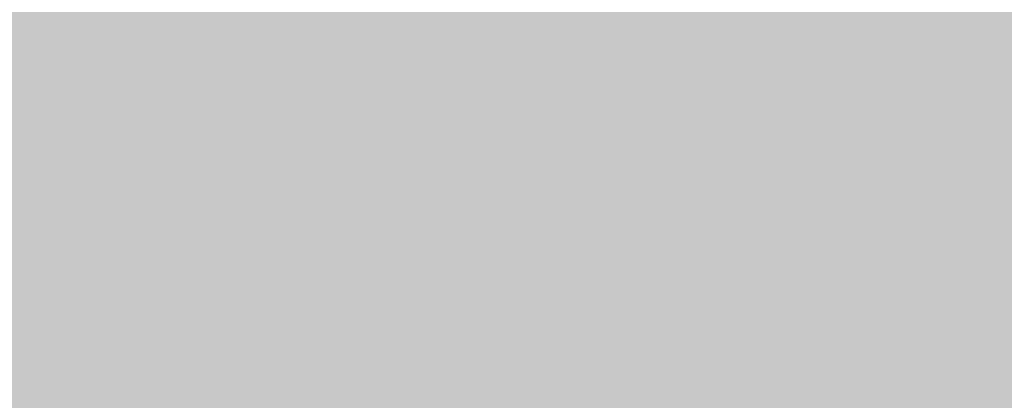
# Model space of a CAD drawing. Units: feet. Extents: x 3168 to 4724, y 827 to 1477.
# Tile 56 of 256: x 3273.139442 to 3273.143144, y 1099.01485 to 1099.016281. Entities that reach past the tile are written whole.
import ezdxf

# ---------------------------------------------------------------- set-up
doc = ezdxf.new("R2010")
doc.units = ezdxf.units.FT
doc.layers.add('A-ELEV', color=7, linetype='Continuous', lineweight=35)
doc.layers.add('A-ELEV-PATT', color=8, linetype='Continuous', lineweight=13)

msp = doc.modelspace()

# ---------------------------------------------------------------- hatches: boundary and pattern name
at = {"layer": 'A-ELEV-PATT'}
h = msp.add_hatch(color=256, dxfattribs=at)
h.dxf.hatch_style = 1
edge = h.paths.add_edge_path()
edge.add_ellipse((3552.9057615, 979.2201412), major_axis=(36.7449243, 0), ratio=0.4848484848, start_angle=0, end_angle=360)
edge = h.paths.add_edge_path()
edge.add_ellipse((3559.8916366, 929.2522824), major_axis=(36.7449243, 0), ratio=0.4848484848, start_angle=0, end_angle=360)
edge = h.paths.add_edge_path()
edge.add_line((3299.3168105, 1198.606081), (3479.9167135, 1198.606081))
edge.add_line((3479.9167135, 1198.606081), (3479.9167135, 1209.8685704))
edge.add_spline(control_points=[(3479.9167135, 1209.8685704), (3464.3011571, 1209.8685704), (3448.6856007, 1209.8685704), (3410.949139, 1209.8685704), (3388.8282339, 1209.8685704), (3355.6468761, 1209.8685704), (3344.5864235, 1209.8685704), (3327.9957446, 1209.8685704), (3322.4655183, 1209.8685704), (3314.1701788, 1209.8685704), (3311.4050657, 1209.8685704), (3307.257396, 1209.8685704), (3305.8748394, 1209.8685704), (3303.8010045, 1209.8685704), (3303.1097262, 1209.8685704), (3302.0728088, 1209.8685704), (3301.7271697, 1209.8685704), (3301.2087109, 1209.8685704), (3301.0358914, 1209.8685704), (3300.776662, 1209.8685704), (3300.6902522, 1209.8685704), (3300.5606376, 1209.8685704), (3300.5174327, 1209.8685704), (3300.4526253, 1209.8685704), (3300.4310229, 1209.8685704), (3300.3986192, 1209.8685704), (3300.387818, 1209.8685704), (3300.3662155, 1209.8685704), (3300.3456757, 1209.8685704), (3300.3455476, 1209.8685704), (3300.345505, 1209.8685704), (3300.3433041, 1209.8685704), (3300.341146, 1209.8685707), (3300.337909, 1209.8685714), (3300.33683, 1209.8685718), (3300.3339422, 1209.8685728), (3300.3321334, 1209.8685736), (3300.3255154, 1209.8685773), (3300.3207065, 1209.8685812), (3300.3109248, 1209.8685917), (3300.305952, 1209.8685984), (3300.2905113, 1209.8686233), (3300.2800452, 1209.8686461), (3300.2324255, 1209.868777), (3300.1952979, 1209.868954), (3299.9510684, 1209.8706077), (3299.7448244, 1209.8743259), (3299.4368271, 1209.8832566), (3299.3343894, 1209.8867924), (3299.181079, 1209.8929197), (3299.1300333, 1209.8950994), (3298.6522171, 1209.9168011), (3298.2294605, 1209.9457176), (3297.6016312, 1210.0023671), (3297.3934043, 1210.0234637), (3297.082652, 1210.058309), (3296.9793324, 1210.0704575), (3296.2929541, 1210.1548606), (3295.7181475, 1210.2433556), (3294.8687167, 1210.3988504), (3294.5876997, 1210.4544779), (3294.1693407, 1210.5433488), (3294.0304153, 1210.5738777), (3291.7071487, 1211.1012), (3289.6535901, 1211.8134353), (3285.7762586, 1213.5639876), (3283.9514101, 1214.6034778), (3280.512159, 1216.9800798), (3278.8972407, 1218.3175918), (3276.3799143, 1220.829489), (3275.4160415, 1221.9177379), (3274.0393421, 1223.7076996), (3273.5810428, 1224.3495346), (3273.1432283, 1225.0163162)], knot_values=[39.119033, 39.119033, 39.119033, 39.119033, 39.286353, 39.286353, 39.523379, 39.523379, 39.641892, 39.641892, 39.701148, 39.701148, 39.730777, 39.730777, 39.745591, 39.745591, 39.752998, 39.752998, 39.756701, 39.756701, 39.758553, 39.758553, 39.759479, 39.759479, 39.759942, 39.759942, 39.760173, 39.760173, 39.760289, 39.760289, 39.760405, 39.760405, 39.760463, 39.760463, 39.763389, 39.763389, 39.764851, 39.764851, 39.767304, 39.767304, 39.773825, 39.773825, 39.78057, 39.78057, 39.79477, 39.79477, 39.845194, 39.845194, 40.126715, 40.126715, 40.267476, 40.267476, 40.337856, 40.337856, 40.927023, 40.927023, 41.221606, 41.221606, 41.368898, 41.368898, 42.202622, 42.202622, 42.619485, 42.619485, 42.827916, 42.827916, 46.118323, 46.118323, 49.408731, 49.408731, 52.699139, 52.699139, 54.927489, 54.927489, 56.104228, 56.104228, 56.104228, 56.104228], weights=[1, 1, 1, 1, 1, 1, 1, 1, 1, 1, 1, 1, 1, 1, 1, 1, 1, 1, 1, 1, 1, 1, 1, 1, 1, 1, 1, 1, 1, 1, 1, 1, 1, 1, 1, 1, 1, 1, 1, 1, 1, 1, 1, 1, 1, 1, 1, 1, 1, 1, 1, 1, 1, 1, 1, 1, 1, 1, 1, 1, 1, 1, 1, 1, 1, 1, 1, 1, 1, 1, 1, 1, 1, 1], degree=3, periodic=0)
edge.add_line((3273.1432283, 1225.0163162), (3273.1432283, 1099.0163162))
edge.add_line((3273.1432283, 1099.0163162), (3299.3168105, 1099.0163162))
edge.add_line((3299.3168105, 1099.0163162), (3299.3168105, 1198.606081))
edge = h.paths.add_edge_path()
edge.add_line((3304.7584434, 1324.15806), (3479.9167135, 1324.15806))
edge.add_line((3479.9167135, 1324.15806), (3479.9167135, 1335.7146184))
edge.add_line((3479.9167135, 1335.7146184), (3269.1616284, 1335.7146184))
edge.add_spline(control_points=[(3269.1616284, 1335.7146184), (3264.0242315, 1335.7146184), (3258.364118, 1328.9581888), (3259.2643109, 1323.9002743)], knot_values=[0, 0, 0, 0, 15.412191, 15.412191, 15.412191, 15.412191], degree=3, periodic=0)
edge.add_line((3259.2643109, 1323.9002743), (3265.5168487, 1288.7691348))
edge.add_line((3265.5168487, 1288.7691348), (3275.2651026, 1261.5456259))
edge.add_line((3275.2651026, 1261.5456259), (3304.7584434, 1261.5456259))
edge.add_line((3304.7584434, 1261.5456259), (3304.7584434, 1324.15806))
h = msp.add_hatch(color=256, dxfattribs=at)
h.dxf.hatch_style = 1
h.paths.add_polyline_path([(3384.5252473, 1099.0163162), (3335.0291678, 1099.0163162), (3299.3168105, 1099.0163162), (3273.1432283, 1099.0163162), (3217.5653642, 1099.0163162), (3168.0692847, 827.1162598), (3335.0291678, 827.1162598)])

# ---------------------------------------------------------------- linework, layer by layer
at = {"layer": 'A-ELEV'}
msp.add_open_spline([(3808.5202001, 1099.0163162), (3808.5202001, 1141.413235), (3808.5202001, 1183.8101539), (3808.5202001, 1226.6353244), (3808.5202001, 1227.0635761), (3808.5202001, 1227.4918279), (3811.491871, 1248.9946729), (3814.463542, 1270.497518), (3817.4652299, 1292.2175635), (3817.4952467, 1292.434764), (3817.5252636, 1292.6519644), (3817.5728014, 1310.1067483), (3817.6203393, 1327.5615322), (3817.6678771, 1345.0163162), (3817.6678771, 1345.4579619), (3817.6678771, 1345.8996077), (3817.6678771, 1346.4560466), (3817.6678771, 1346.5708398), (3817.6678771, 1346.7528874), (3817.6678771, 1346.8201418), (3817.6678771, 1346.9348705), (3817.6678771, 1346.9823447), (3817.6678771, 1347.0385872), (3817.6678771, 1347.0473556), (3817.6678771, 1347.0736607), (3817.667877, 1347.0593025), (3817.6678766, 1347.0615455), (3817.6678764, 1347.0626669), (3817.6678754, 1347.0660311), (3817.6678743, 1347.0682738), (3817.6678701, 1347.0750012), (3817.667866, 1347.0794856), (3817.6678493, 1347.0929368), (3817.6678325, 1347.1019019), (3817.6677657, 1347.1287896), (3817.6676988, 1347.1467049), (3817.6674317, 1347.2004211), (3817.6671649, 1347.2361922), (3817.6661003, 1347.3433849), (3817.6650383, 1347.4146859), (3817.6608124, 1347.6280949), (3817.6566084, 1347.7697085), (3817.6399698, 1348.1924868), (3817.6235091, 1348.4715855), (3817.5590944, 1349.3000666), (3817.4961208, 1349.8405878), (3817.2554319, 1351.4241561), (3817.0263177, 1352.4287852), (3816.3068713, 1354.8889138), (3815.7437452, 1356.2687272), (3814.4639586, 1358.8192105), (3813.7464132, 1359.9909676), (3812.1958378, 1362.1723433), (3811.3622453, 1363.1821237), (3809.5888357, 1365.0690087), (3808.6488164, 1365.9461052), (3806.6542623, 1367.5796162), (3805.5997024, 1368.336154), (3803.3528906, 1369.7223272), (3802.1605354, 1370.352386), (3799.6008131, 1371.4535864), (3798.2326878, 1371.9254812), (3795.2800838, 1372.6346239), (3793.6931479, 1372.8720685), (3791.8694413, 1372.9264797), (3791.7408615, 1372.9292203), (3791.3533713, 1372.9341014), (3791.0927074, 1372.9329013), (3790.3041163, 1372.9150676), (3789.7695426, 1372.8841946), (3789.20919, 1372.8302363), (3789.1906217, 1372.8284241), (3789.1348916, 1372.8229123), (3789.097705, 1372.8191375), (3789.0484446, 1372.8140077), (3789.0364001, 1372.8127432), (3789.0002562, 1372.808918), (3788.9761468, 1372.8063255), (3788.9494049, 1372.8034042), (3788.9467858, 1372.8031177), (3788.9425667, 1372.8026552), (3788.9409669, 1372.8024797), (3788.9385718, 1372.8022166), (3788.9377765, 1372.8021292), (3788.9353908, 1372.8018669), (3788.8675349, 1372.7944024), (3788.7568665, 1372.7822285), (3788.7015323, 1372.7761415), (3788.5355297, 1372.7578805), (3788.4248612, 1372.7457065), (3788.092856, 1372.7091846), (3787.8715192, 1372.6848366), (3787.2075086, 1372.6117927), (3786.764835, 1372.5630968), (3785.436814, 1372.417009), (3784.5514666, 1372.3196171), (3781.8954246, 1372.0274416), (3780.1247299, 1371.8326579), (3774.8126458, 1371.2483067), (3771.2712564, 1370.8587393), (3760.6470883, 1369.6900371), (3753.5643095, 1368.9109022), (3732.3159732, 1366.5734977), (3718.1504157, 1365.015228), (3694.0067577, 1362.3593262), (3684.0286573, 1361.2616941), (3674.0505568, 1360.1640619), (3664.6006617, 1360.1640619), (3655.1507666, 1360.1640619), (3626.8010812, 1360.1640619), (3607.9012909, 1360.1640619), (3551.2019201, 1360.1640619), (3513.4023395, 1360.1640619), (3467.7251817, 1360.1640619), (3459.8476045, 1360.1640619), (3436.2148727, 1360.1640619), (3420.4597182, 1360.1640619), (3373.1942547, 1360.1640619), (3341.6839457, 1360.1640619), (3302.8481616, 1360.1640619), (3295.5226865, 1360.1640619), (3286.0382916, 1360.1640619), (3283.8793719, 1360.1640619), (3277.4026128, 1360.1640619), (3273.0847733, 1360.1640619), (3267.7328511, 1360.1640619), (3266.6987684, 1360.1640619), (3263.5965201, 1360.1640619), (3261.5283546, 1360.1640619), (3259.2369429, 1360.1640619), (3259.0136967, 1360.1640619), (3258.3439582, 1360.1640619), (3257.8974658, 1360.1640619), (3257.4309979, 1360.1640619), (3257.4110224, 1360.1640619), (3257.3705735, 1360.1640619), (3257.3754695, 1360.1640619), (3257.3745975, 1360.1640619), (3257.3739371, 1360.1640618), (3257.3719559, 1360.1640616), (3257.3706351, 1360.1640613), (3257.366673, 1360.16406), (3257.3640318, 1360.1640586), (3257.3561088, 1360.1640529), (3257.3508277, 1360.1640469), (3257.3349869, 1360.1640226), (3257.3244299, 1360.163998), (3257.2927692, 1360.1638987), (3257.2716761, 1360.1637987), (3257.208439, 1360.1633975), (3257.1663373, 1360.1629953), (3257.0402058, 1360.1613882), (3256.9563493, 1360.1597827), (3256.705504, 1360.1533932), (3256.53924, 1360.1470361), (3256.0435702, 1360.1219156), (3255.717296, 1360.0971018), (3254.7524458, 1360.0004808), (3254.1279679, 1359.906513), (3252.1800666, 1359.5253322), (3250.9415739, 1359.1439911), (3248.6701751, 1358.2432905), (3247.6357388, 1357.7238339), (3245.7326321, 1356.6034712), (3244.8633884, 1356.0020595), (3243.2531076, 1354.7428655), (3242.511972, 1354.0847309), (3240.7510518, 1352.3447812), (3239.8009609, 1351.229574), (3238.0877694, 1348.8724402), (3237.3246853, 1347.6303552), (3235.9825098, 1344.9716321), (3235.4022051, 1343.554907), (3234.5910812, 1340.8154577), (3234.3108819, 1339.5435498), (3233.9764902, 1336.8025605), (3233.9221126, 1335.3308771), (3234.1489156, 1332.5912693), (3234.3495287, 1331.3672011), (3234.7198926, 1329.9993668), (3234.7524228, 1329.8833616), (3234.853619, 1329.5347966), (3234.9258923, 1329.301685), (3235.0248359, 1329.0025524), (3235.0469235, 1328.936928), (3235.0776388, 1328.8472393), (3235.0859239, 1328.8231979), (3235.1109389, 1328.7510642), (3235.1278282, 1328.7029624), (3235.1479919, 1328.6462418), (3235.1510592, 1328.6376324), (3235.1560959, 1328.6235265), (3235.1580611, 1328.6180301), (3235.1602094, 1328.6120302), (3235.1656119, 1328.596943), (3235.1800989, 1328.556486), (3235.190263, 1328.5281009), (3235.2207556, 1328.4429457), (3235.241084, 1328.3861755), (3235.3020692, 1328.215865), (3235.3427259, 1328.1023247), (3235.4646962, 1327.7617038), (3235.5460097, 1327.5346232), (3235.7899503, 1326.8533813), (3235.9525774, 1326.39922), (3236.4404586, 1325.0367362), (3236.7657127, 1324.1284137), (3237.7414751, 1321.4034462), (3238.3919833, 1319.5868011), (3240.3435081, 1314.136866), (3241.6445245, 1310.503576), (3245.547574, 1299.6037058), (3248.149607, 1292.3371257), (3255.955706, 1270.5373853), (3261.1597719, 1256.004225), (3267.3876177, 1238.6120011), (3268.4113975, 1235.7529374), (3269.5103781, 1232.6838639), (3269.5855789, 1232.473854), (3269.7066118, 1232.1358507), (3269.752444, 1232.0078573), (3269.8273289, 1231.7987296), (3269.8563817, 1231.7175953), (3269.9063247, 1231.5781217), (3269.927215, 1231.5197823), (3269.9724682, 1231.3934057), (3269.9968311, 1231.3253685), (3270.0265026, 1231.2425062), (3270.0318112, 1231.2276812), (3270.0402823, 1231.2040243), (3270.0392242, 1231.2069792), (3270.0393595, 1231.2066014), (3270.0394271, 1231.2064125), (3270.0396301, 1231.2058458), (3270.0397654, 1231.205468), (3270.0401713, 1231.2043346), (3270.040442, 1231.2035791), (3270.041254, 1231.2013125), (3270.0417955, 1231.1998016), (3270.0434203, 1231.195269), (3270.044504, 1231.1922477), (3270.0477563, 1231.1831849), (3270.0499263, 1231.1771446), (3270.0564418, 1231.1590283), (3270.0607927, 1231.146957), (3270.0738674, 1231.1107614), (3270.0826128, 1231.0866558), (3270.1089357, 1231.0144129), (3270.1265997, 1230.9663498), (3270.1799341, 1230.8224568), (3270.2159467, 1230.7269233), (3270.3253234, 1230.4415078), (3270.4000257, 1230.2528107), (3270.6292491, 1229.6914436), (3270.7888829, 1229.3235005), (3271.2864875, 1228.2383194), (3271.6430996, 1227.5397546), (3272.7758592, 1225.515277), (3273.6141694, 1224.2605021), (3275.4160415, 1221.9177379), (3276.3799143, 1220.829489), (3278.8972407, 1218.3175918), (3280.512159, 1216.9800798), (3283.9514101, 1214.6034778), (3285.7762586, 1213.5639876), (3289.6535901, 1211.8134353), (3291.7071487, 1211.1012), (3294.0304153, 1210.5738777), (3294.1693407, 1210.5433488), (3294.5876997, 1210.4544779), (3294.8687167, 1210.3988504), (3295.7181475, 1210.2433556), (3296.2929541, 1210.1548606), (3296.9793324, 1210.0704575), (3297.082652, 1210.058309), (3297.3934043, 1210.0234637), (3297.6016312, 1210.0023671), (3298.2294605, 1209.9457176), (3298.6522171, 1209.9168011), (3299.1300333, 1209.8950994), (3299.181079, 1209.8929197), (3299.3343894, 1209.8867924), (3299.4368271, 1209.8832566), (3299.7448244, 1209.8743259), (3299.9510684, 1209.8706077), (3300.1952979, 1209.868954), (3300.2324255, 1209.868777), (3300.2800452, 1209.8686461), (3300.2905113, 1209.8686233), (3300.305952, 1209.8685984), (3300.3109248, 1209.8685917), (3300.3207065, 1209.8685812), (3300.3255154, 1209.8685773), (3300.3321334, 1209.8685736), (3300.3339422, 1209.8685728), (3300.33683, 1209.8685718), (3300.337909, 1209.8685714), (3300.341146, 1209.8685707), (3300.3433041, 1209.8685704), (3300.345505, 1209.8685704), (3300.3455476, 1209.8685704), (3300.3456757, 1209.8685704), (3300.3662155, 1209.8685704), (3300.387818, 1209.8685704), (3300.3986192, 1209.8685704), (3300.4310229, 1209.8685704), (3300.4526253, 1209.8685704), (3300.5174327, 1209.8685704), (3300.5606376, 1209.8685704), (3300.6902522, 1209.8685704), (3300.776662, 1209.8685704), (3301.0358914, 1209.8685704), (3301.2087109, 1209.8685704), (3301.7271697, 1209.8685704), (3302.0728088, 1209.8685704), (3303.1097262, 1209.8685704), (3303.8010045, 1209.8685704), (3305.8748394, 1209.8685704), (3307.257396, 1209.8685704), (3311.4050657, 1209.8685704), (3314.1701788, 1209.8685704), (3322.4655183, 1209.8685704), (3327.9957446, 1209.8685704), (3344.5864235, 1209.8685704), (3355.6468761, 1209.8685704), (3388.8282339, 1209.8685704), (3410.949139, 1209.8685704), (3477.3118546, 1209.8685704), (3521.553665, 1209.8685704), (3566.8361836, 1209.8685704), (3567.8768919, 1209.8685704), (3570.9990167, 1209.8685704), (3573.0804332, 1209.8685704), (3575.7813964, 1209.8685704), (3576.4009432, 1209.8685704), (3577.2958211, 1209.8685704), (3577.5711523, 1209.8685704), (3578.3971458, 1209.8685704), (3578.9478081, 1209.8685704), (3579.7564907, 1209.8685704), (3580.0145108, 1209.8685704), (3580.3427367, 1209.8685704), (3580.3268649, 1209.8685704), (3580.3271702, 1209.8685704), (3580.3273229, 1209.8685704), (3580.3277809, 1209.8685704), (3580.3280863, 1209.8685704), (3580.3290024, 1209.8685703), (3580.3296132, 1209.8685702), (3580.3314455, 1209.8685699), (3580.332667, 1209.8685697), (3580.336332, 1209.8685685), (3580.3387755, 1209.8685674), (3580.3461066, 1209.8685629), (3580.350995, 1209.8685584), (3580.3656627, 1209.8685402), (3580.3754446, 1209.868522), (3580.4048012, 1209.8684493), (3580.4243863, 1209.8683764), (3580.4831833, 1209.8680848), (3580.5224371, 1209.8677929), (3580.6403612, 1209.8666242), (3580.7191947, 1209.8654543), (3580.9563152, 1209.8607663), (3581.1152222, 1209.85607), (3581.5941635, 1209.8372298), (3581.9164188, 1209.8183314), (3582.8899466, 1209.7424284), (3583.547986, 1209.6661692), (3585.5318268, 1209.3606172), (3586.8672159, 1209.0538859), (3589.4715454, 1208.2524717), (3590.7402412, 1207.7578521), (3591.9954511, 1207.1588024), (3592.057809, 1207.1287398), (3592.2442418, 1207.0379536), (3592.3676757, 1206.9766317), (3592.73528, 1206.7903591), (3592.9767518, 1206.663101), (3593.2445387, 1206.5164414), (3593.2747313, 1206.4998248), (3593.3651153, 1206.4498388), (3593.4251129, 1206.4163333), (3593.6043138, 1206.3152851), (3593.7227254, 1206.2472105), (3593.8572122, 1206.1683978), (3593.8743621, 1206.1583193), (3593.925741, 1206.1280407), (3593.9598989, 1206.1077976), (3594.0620855, 1206.0468991), (3594.1298272, 1206.0060745), (3594.2084359, 1205.9581709), (3594.2196829, 1205.9513043), (3594.253391, 1205.9306863), (3594.2758193, 1205.9169166), (3594.3429716, 1205.8755358), (3594.3875633, 1205.8478526), (3594.4336161, 1205.8190499), (3594.4352559, 1205.818024), (3594.4401746, 1205.8149461), (3594.4434527, 1205.8128936), (3594.4471229, 1205.8105944), (3594.4475159, 1205.8103482), (3594.4486949, 1205.8096095), (3594.4494808, 1205.8091171), (3594.4503663, 1205.8085621), (3594.4504658, 1205.8084998), (3594.4506003, 1205.8084155), (3594.4673993, 1205.7978872), (3594.4932689, 1205.7816741), (3594.5062037, 1205.7735675), (3594.5450081, 1205.7492479), (3594.5708778, 1205.7330348), (3594.6484866, 1205.6843956), (3594.7002258, 1205.6519694), (3594.8554436, 1205.5546909), (3594.958922, 1205.4898386), (3595.2693574, 1205.2952816), (3595.4763144, 1205.1655769), (3596.0971852, 1204.7764629), (3596.5110991, 1204.5170536), (3597.7528407, 1203.7388256), (3598.5806685, 1203.220007), (3601.0641518, 1201.663551), (3602.7198073, 1200.6259137), (3607.686774, 1197.5130018), (3610.998085, 1195.4377272), (3620.9320182, 1189.2119034), (3627.5546404, 1185.0613542), (3647.4225068, 1172.6097066), (3660.6677511, 1164.3086082), (3700.403484, 1139.405313), (3726.8939725, 1122.8031161), (3757.2057154, 1103.8060516), (3761.0269697, 1101.4111839), (3764.848224, 1099.0163162), (3745.3282713, 1099.0163162), (3725.8083186, 1099.0163162), (3706.288366, 1099.0163162), (3706.288366, 1108.4532371), (3706.288366, 1117.890158), (3706.288366, 1127.3270789), (3710.7507544, 1127.3270789), (3715.2131428, 1127.3270789), (3719.6755312, 1127.3270789)], degree=3, knots=[0, 0, 0, 0, 0.982037, 0.982037, 0.991957, 0.991957, 0.991957, 1.966522, 1.966522, 1.976367, 1.976367, 1.976367, 2.976367, 2.976367, 2.976367, 3.00169, 3.00169, 3.008272, 3.008272, 3.012129, 3.012129, 3.014851, 3.014851, 3.015353, 3.015353, 3.016359, 3.016359, 3.017365, 3.017365, 3.019376, 3.019376, 3.023398, 3.023398, 3.031442, 3.031442, 3.047531, 3.047531, 3.079708, 3.079708, 3.144063, 3.144063, 3.272772, 3.272772, 3.53019, 3.53019, 4.045026, 4.045026, 5.074698, 5.074698, 6.700878, 6.700878, 8.327058, 8.327058, 9.953238, 9.953238, 11.579418, 11.579418, 13.205598, 13.205598, 14.831778, 14.831778, 16.457958, 16.457958, 18.084138, 18.084138, 18.206872, 18.206872, 18.45234, 18.45234, 18.943275, 18.943275, 18.960093, 18.960093, 18.993729, 18.993729, 19.00461, 19.00461, 19.026374, 19.026374, 19.028737, 19.028737, 19.03018, 19.03018, 19.030897, 19.030897, 19.032332, 19.032332, 19.033766, 19.033766, 19.036636, 19.036636, 19.042374, 19.042374, 19.053851, 19.053851, 19.076805, 19.076805, 19.122714, 19.122714, 19.21453, 19.21453, 19.398163, 19.398163, 19.765429, 19.765429, 20.024128, 20.024128, 20.024128, 20.092031, 20.092031, 20.227836, 20.227836, 20.499446, 20.499446, 20.556051, 20.556051, 20.66926, 20.66926, 20.895678, 20.895678, 20.948316, 20.948316, 20.963829, 20.963829, 20.994855, 20.994855, 21.002285, 21.002285, 21.017146, 21.017146, 21.01875, 21.01875, 21.021959, 21.021959, 21.022102, 21.022102, 21.022249, 21.022249, 21.022708, 21.022708, 21.023627, 21.023627, 21.025464, 21.025464, 21.029138, 21.029138, 21.036486, 21.036486, 21.051183, 21.051183, 21.080575, 21.080575, 21.139361, 21.139361, 21.256932, 21.256932, 21.492073, 21.492073, 21.962356, 21.962356, 23.01002, 23.01002, 24.057684, 24.057684, 25.105348, 25.105348, 26.153011, 26.153011, 27.776787, 27.776787, 29.400562, 29.400562, 31.024337, 31.024337, 32.278801, 32.278801, 33.533265, 33.533265, 34.467568, 34.467568, 34.553971, 34.553971, 34.726776, 34.726776, 34.775309, 34.775309, 34.793079, 34.793079, 34.82862, 34.82862, 34.834979, 34.834979, 34.839039, 34.839039, 34.839411, 34.839411, 34.840285, 34.840285, 34.842034, 34.842034, 34.845531, 34.845531, 34.852525, 34.852525, 34.866512, 34.866512, 34.894488, 34.894488, 34.950439, 34.950439, 35.062342, 35.062342, 35.286147, 35.286147, 35.733758, 35.733758, 35.821815, 35.821815, 35.828283, 35.828283, 35.832225, 35.832225, 35.834724, 35.834724, 35.836521, 35.836521, 35.838617, 35.838617, 35.839073, 35.839073, 35.839345, 35.839345, 35.839617, 35.839617, 35.840161, 35.840161, 35.841249, 35.841249, 35.843425, 35.843425, 35.847778, 35.847778, 35.856482, 35.856482, 35.873891, 35.873891, 35.908709, 35.908709, 35.978345, 35.978345, 36.117617, 36.117617, 36.396161, 36.396161, 36.953248, 36.953248, 38.067423, 38.067423, 40.295772, 40.295772, 42.524122, 42.524122, 45.81453, 45.81453, 49.104937, 49.104937, 52.395345, 52.395345, 52.603776, 52.603776, 53.020639, 53.020639, 53.854363, 53.854363, 54.001655, 54.001655, 54.296238, 54.296238, 54.885405, 54.885405, 54.955785, 54.955785, 55.096546, 55.096546, 55.378067, 55.378067, 55.42849, 55.42849, 55.442691, 55.442691, 55.449436, 55.449436, 55.455957, 55.455957, 55.458409, 55.458409, 55.459872, 55.459872, 55.462798, 55.462798, 55.462856, 55.462856, 55.462972, 55.462972, 55.463088, 55.463088, 55.463319, 55.463319, 55.463782, 55.463782, 55.464708, 55.464708, 55.46656, 55.46656, 55.470263, 55.470263, 55.47767, 55.47767, 55.492484, 55.492484, 55.522112, 55.522112, 55.581369, 55.581369, 55.699882, 55.699882, 55.936907, 55.936907, 56.410959, 56.410959, 56.42211, 56.42211, 56.444413, 56.444413, 56.451051, 56.451051, 56.454001, 56.454001, 56.459901, 56.459901, 56.462666, 56.462666, 56.463418, 56.463418, 56.464171, 56.464171, 56.465675, 56.465675, 56.468684, 56.468684, 56.474702, 56.474702, 56.486738, 56.486738, 56.51081, 56.51081, 56.558955, 56.558955, 56.655243, 56.655243, 56.847821, 56.847821, 57.232975, 57.232975, 58.003284, 58.003284, 59.543901, 59.543901, 62.625137, 62.625137, 68.787607, 68.787607, 74.950078, 74.950078, 75.27336, 75.27336, 75.919923, 75.919923, 77.213051, 77.213051, 77.377769, 77.377769, 77.707206, 77.707206, 78.366079, 78.366079, 78.462532, 78.462532, 78.655436, 78.655436, 79.041245, 79.041245, 79.105735, 79.105735, 79.234714, 79.234714, 79.492672, 79.492672, 79.502197, 79.502197, 79.521249, 79.521249, 79.523534, 79.523534, 79.528103, 79.528103, 79.528682, 79.528682, 79.528885, 79.528885, 79.529089, 79.529089, 79.529495, 79.529495, 79.530308, 79.530308, 79.531935, 79.531935, 79.535187, 79.535187, 79.541693, 79.541693, 79.554704, 79.554704, 79.580725, 79.580725, 79.632769, 79.632769, 79.736856, 79.736856, 79.94503, 79.94503, 80.361377, 80.361377, 80.421435, 80.421435, 80.421435, 81.421435, 81.421435, 81.421435, 82.421435, 82.421435, 82.421435, 83.421435, 83.421435, 83.421435, 83.421435], dxfattribs=at)

doc.saveas('drawing.dxf')
